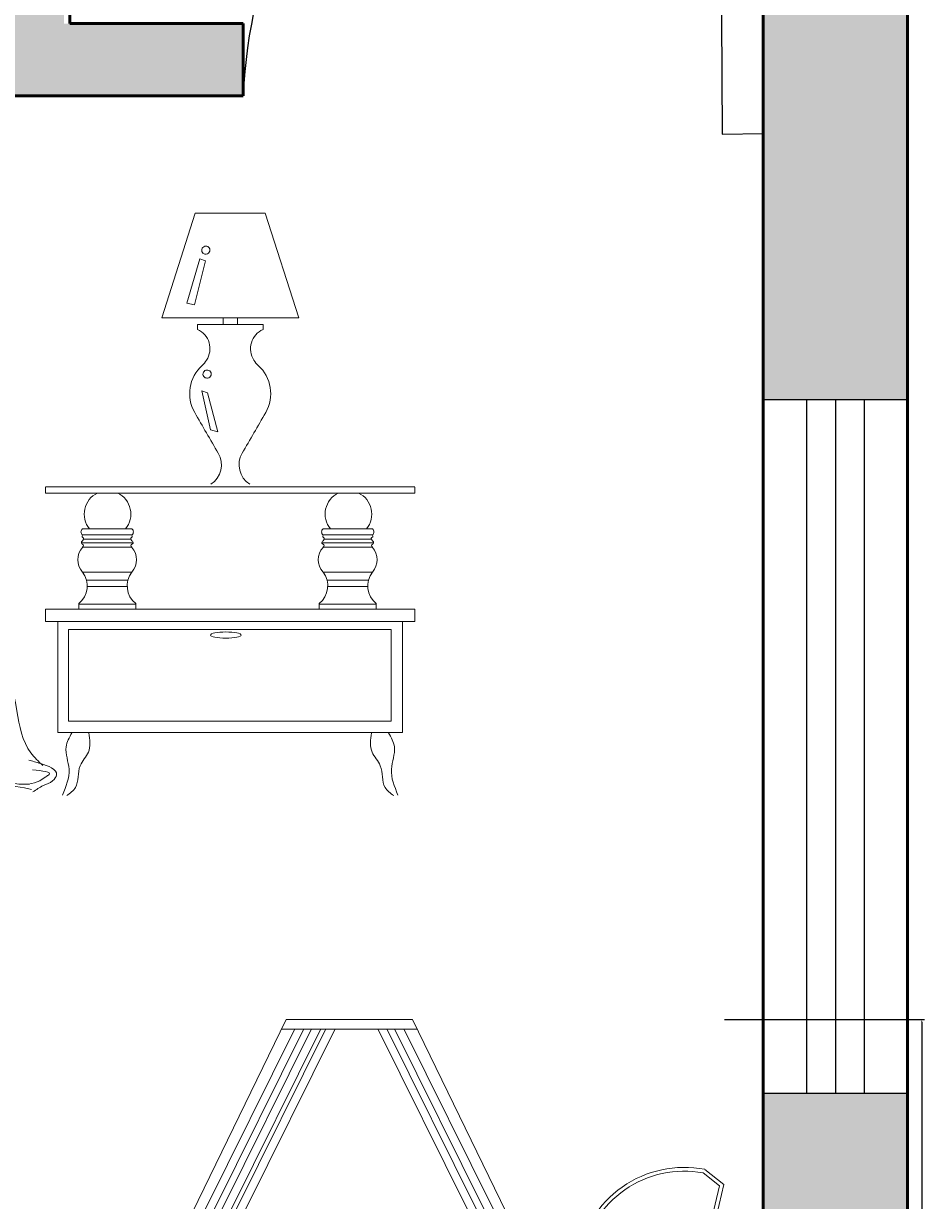
# Model space of a CAD drawing. Units: inches. Extents: x 1771 to 3025, y 319 to 889.
# Tile 11 of 35: x 2040 to 2102, y 713 to 795. Entities that reach past the tile are written whole.
import ezdxf

# ---------------------------------------------------------------- set-up
doc = ezdxf.new("R2010")
doc.units = ezdxf.units.IN
doc.header["$MEASUREMENT"] = 0
doc.set_wipeout_variables(frame=1)
for name, color, linetype, lineweight in [('A-ANNO-DIMS', 2, 'Continuous', 18), ('A-DOOR', 4, 'Continuous', 25), ('A-FURN', 8, 'Continuous', 18), ('A-GLAZ', 40, 'Continuous', 25), ('A-WALL', 7, 'Continuous', 50), ('A-WALL-PATT', 254, 'Continuous', 13)]:
    doc.layers.add(name, color=color, linetype=linetype, lineweight=lineweight)
doc.styles.get("Standard").update_dxf_attribs({"font": 'arial.ttf'})
doc.dimstyles.get("Standard").update_dxf_attribs({"dimtxt": 0.18, "dimasz": 0.18, "dimexe": 0.18, "dimexo": 0.0625, "dimgap": 0.09, "dimtad": 0, "dimtih": 1, "dimtoh": 1, "dimdec": 4, "dimzin": 0, "dimdsep": 46, "dimtxsty": 'Standard', "dimcen": 0.09, "dimadec": 0, "dimazin": 0, "dimtfac": 1, "dimtdec": 4, "dimtofl": 0, "dimtmove": 0, "dimatfit": 3, "dimfxl": 1, "dimtolj": 1, "dimtzin": 0, "dimarcsym": 0})

# ---------------------------------------------------------------- blocks, each defined once
blk = doc.blocks.new('A$C3F6F0378')
for p, q in [((2294.6, 774.2), (2348.7, 943.6)), ((2462.2, 943.6), (2348.7, 943.6)), ((2516.4, 774.2), (2462.2, 943.6)), ((2335.1, 797.8), (2356.3, 869.3)), ((2365.5, 866.2), (2347.3, 794.8)), ((2356.3, 869.3), (2365.5, 866.2)), ((2347.3, 794.8), (2335.1, 797.8)), ((2516.4, 774.2), (2294.6, 774.2)), ((2352.3, 763), (2352.3, 755.2)), ((2352.3, 763), (2352.3, 755.2)), ((2458.6, 763), (2352.3, 763)), ((2393.8, 774.2), (2393.8, 763)), ((2417.1, 763), (2393.8, 763)), ((2417.1, 774.2), (2417.1, 763)), ((2458.6, 763), (2458.6, 755.2)), ((2458.6, 763), (2458.6, 755.2)), ((2359.5, 655.6), (2368.6, 652.5)), ((2373.2, 592.3), (2359.5, 655.6)), ((2368.6, 652.5), (2385.4, 589.2)), ((2385.4, 589.2), (2373.2, 592.3)), ((2704.5, 500), (2106.1, 500)), ((2106.1, 499.7), (2106.1, 489.7)), ((2704.5, 499.7), (2704.5, 489.7)), ((2704.5, 490), (2106.1, 490)), ((2246.1, 432.2), (2166.1, 432.2)), ((2246.1, 432.2), (2166.1, 432.2)), ((2246.1, 422.2), (2166.1, 422.2)), ((2635.9, 432.2), (2555.9, 432.2)), ((2635.9, 432.2), (2555.9, 432.2)), ((2635.9, 422.2), (2555.9, 422.2)), ((2248, 409.3), (2164.1, 409.3)), ((2246.1, 402.2), (2166.1, 402.2)), ((2244.2, 415.4), (2167.9, 415.4)), ((2637.9, 409.3), (2554, 409.3)), ((2635.9, 402.2), (2555.9, 402.2)), ((2634.1, 415.4), (2557.7, 415.4)), ((2246.1, 362.2), (2166.1, 362.2)), ((2239.7, 349.2), (2172.4, 349.2)), ((2635.9, 362.2), (2555.9, 362.2)), ((2629.6, 349.2), (2562.2, 349.2)), ((2238.5, 338.7), (2173.6, 338.7)), ((2628.4, 338.7), (2563.5, 338.7)), ((2159.8, 311), (2159.8, 302.2)), ((2252.3, 310.3), (2159.8, 310.3)), ((2252.3, 311), (2252.3, 302.2)), ((2549.7, 311), (2549.7, 302.2)), ((2642.2, 310.3), (2549.7, 310.3)), ((2642.2, 311), (2642.2, 302.2)), ((2106.1, 302.2), (2106.1, 282.2)), ((2704.5, 302.2), (2106.1, 302.2)), ((2186.1, 302.2), (2226.1, 302.2)), ((2186.1, 302.2), (2236.1, 302.2)), ((2575.9, 302.2), (2615.9, 302.2)), ((2575.9, 302.2), (2625.9, 302.2)), ((2704.5, 282.2), (2704.5, 302.2)), ((2704.5, 282.2), (2106.1, 282.2)), ((2126.1, 282.2), (2126.1, 102.2)), ((2143.3, 268.9), (2666.3, 268.9)), ((2143.3, 120.8), (2143.3, 268.9)), ((2666.3, 268.9), (2666.3, 120.8)), ((2684.5, 102.2), (2684.5, 282.2)), ((2666.3, 120.8), (2143.3, 120.8)), ((2126.1, 102.2), (2684.5, 102.2))]:
    blk.add_line(p, q)
for centre, radius, start, end in [((2365.7, 883.6), 6.48, 168.6084, 233.2112), ((2365.7, 883.6), 6.49, 104.0344, 168.6084), ((2365.7, 883.5), 6.42, 233.2112, 255.9722), ((2366.1, 883.6), 6.51, 78.6968, 107.1924), ((2365.7, 883.8), 6.69, 255.9722, 278.2688), ((2365.7, 883.9), 6.81, 278.2688, 342.9026), ((2366.1, 883.7), 6.5, 50.1648, 78.6968), ((2366.2, 883.8), 6.35, 342.9026, 50.1648), ((2338.7, 724.1), 33.9, 326.6744, 66.3416), ((2472.2, 724.1), 33.9, 113.6584, 213.3256), ((2337, 722.3), 34.4, 312.0366, 330.6067), ((2473.8, 722.3), 34.4, 209.3933, 227.9634), ((2401.2, 651.2), 61.5, 132.0366, 209.8723), ((2367.7, 682.8), 6.49, 104.0344, 168.6084), ((2368.1, 682.9), 6.51, 78.6968, 107.1924), ((2368.1, 682.9), 6.5, 50.1648, 78.6968), ((2368.2, 683), 6.35, 342.9026, 50.1648), ((2409.6, 651.2), 61.5, 330.1277, 47.9634), ((2367.7, 682.8), 6.48, 168.6084, 233.2112), ((2367.7, 682.8), 6.42, 233.2112, 255.9722), ((2367.8, 683), 6.69, 255.9722, 278.2688), ((2367.8, 683.1), 6.81, 278.2688, 342.9026), ((11218.8, 5715.8), 10230.1, 209.87228, 210.29853), ((-6408, 5715.8), 10230.1, 329.70147, 330.12772), ((2353.9, 535.9), 37.3, 302.5427, 30.2985), ((2457, 535.9), 37.3, 149.7015, 237.4573), ((2206.6, 456.1), 37.8, 115.9414, 219.2084), ((2206.6, 456.1), 37.8, 320.7916, 64.0586), ((2597, 456.1), 37.8, 115.9414, 219.2084), ((2597, 456.1), 37.8, 320.7916, 64.0586), ((2169.8, 427.2), 6.24, 126.78, 233.22), ((2242.3, 427.2), 6.24, 306.78, 53.22), ((2559.7, 427.2), 6.24, 126.78, 233.22), ((2632.2, 427.2), 6.24, 306.78, 53.22), ((2188.1, 382.2), 29.7, 137.7452, 222.2548), ((2224, 382.2), 29.7, 317.7452, 42.2548), ((2577.9, 382.2), 29.7, 137.7452, 222.2548), ((2613.9, 382.2), 29.7, 317.7452, 42.2548), ((2136.7, 339.8), 37, 308.7547, 37.2668), ((2275.4, 339.8), 37, 142.7332, 231.2453), ((2526.5, 339.8), 37, 308.7547, 37.2668), ((2665.3, 339.8), 37, 142.7332, 231.2453)]:
    blk.add_arc(centre, radius, start, end)
blk.add_ellipse((2398.3, 260.1), major_axis=(25, 0), ratio=0.2)
at = {"ltscale": 5}
for points, knots in [([(2101.8, 49), (2094.8, 55.3), (2069.8, 78.1), (2053.9, 172), (2031.7, 287.1), (2023.3, 445.1), (1887.5, 475), (1637.7, 455.3), (1416.4, 458.5), (1314.5, 461.4)], [0, 0, 0, 0, 28.320233, 100.953775, 269.820348, 420.691469, 489.161544, 656.134073, 940.569207, 940.569207, 940.569207, 940.569207]), ([(2079, 57.4), (2084.9, 55.8), (2100.2, 51.8), (2131, 40.6), (2116.7, 21.1), (2101.3, 16.6), (2091, 9.7), (2085.5, 5.9)], [0, 0, 0, 0, 19.937155, 51.57724, 63.193909, 80.21631, 100.09061, 100.09061, 100.09061, 100.09061]), ([(2080.3, 18.4), (2075.6, 18.3), (2062.2, 17.9), (2030.9, 24.9), (1978.8, 41.9), (1919.5, 46.5), (1879.3, 50.9), (1863, 53.1), (1860.4, 51), (1859.9, 50.7)], [0, 0, 0, 0, 14.447875, 40.468341, 96.220884, 181.018327, 216.046098, 224.609189, 226.185962, 226.185962, 226.185962, 226.185962]), ([(2084.9, 41.8), (2100.9, 40.1), (2120.5, 38.1), (2104.4, 29.7), (2095.5, 21.9), (2085.1, 19.8), (2078.6, 18.4)], [0, 0, 0, 0, 28.05485, 34.289435, 45.980108, 65.027556, 65.027556, 65.027556, 65.027556]), ([(2083.5, 9.9), (2082, 10.3), (2061.3, 15.5), (2017.8, 18.7), (1949.9, 25.1), (1893.7, 17), (1853.5, 15.4), (1840.4, 23.1), (1835.5, 26)], [590.079786, 590.079786, 590.079786, 590.079786, 594.646549, 651.888327, 725.747367, 797.841373, 826.274406, 843.189267, 843.189267, 843.189267, 843.189267])]:
    blk.add_open_spline(points, degree=3, knots=knots, dxfattribs=at)
for points, knots in [([(2166.1, 422.2), (2165.6, 421), (2164.6, 418.8), (2169.4, 417.1), (2166.2, 412.9), (2162.3, 408.7), (2169.1, 405.7), (2166.9, 403.1), (2166.1, 402.2)], [0, 0, 0, 0, 3.125, 6.207289, 10.622222, 14.901958, 20.470919, 23.596268, 23.596268, 23.596268, 23.596268]), ([(2246, 422.2), (2246.5, 421), (2247.5, 418.8), (2242.7, 417.1), (2245.9, 412.9), (2249.8, 408.7), (2243, 405.7), (2245.2, 403.1), (2246, 402.2)], [0, 0, 0, 0, 3.125, 6.207289, 10.622222, 14.901958, 20.470919, 23.596268, 23.596268, 23.596268, 23.596268]), ([(2555.9, 422.2), (2555.5, 421), (2554.5, 418.8), (2559.3, 417.1), (2556.1, 412.9), (2552.2, 408.7), (2559, 405.7), (2556.7, 403.1), (2555.9, 402.2)], [0, 0, 0, 0, 3.125, 6.207289, 10.622222, 14.901958, 20.470919, 23.596268, 23.596268, 23.596268, 23.596268]), ([(2635.9, 422.2), (2636.4, 421), (2637.3, 418.8), (2632.5, 417.1), (2635.8, 412.9), (2639.7, 408.7), (2632.8, 405.7), (2635.1, 403.1), (2635.9, 402.2)], [0, 0, 0, 0, 3.125, 6.207289, 10.622222, 14.901958, 20.470919, 23.596268, 23.596268, 23.596268, 23.596268]), ([(2148.9, 101.6), (2144.7, 94.2), (2134.2, 75.7), (2149.9, 40.1), (2139.4, 14.7), (2133.7, 0.9)], [0, 0, 0, 0, 24.696996, 61.099524, 104.177437, 104.177437, 104.177437, 104.177437]), ([(2176.5, 101.6), (2178, 90.6), (2180.7, 70.5), (2155.8, 47.4), (2161.8, 15.4), (2145.9, 4), (2140.4, 0)], [0, 0, 0, 0, 31.35672, 56.935761, 92.890491, 112.386558, 112.386558, 112.386558, 112.386558]), ([(2634.4, 101.6), (2632.9, 90.6), (2630.2, 70.5), (2655.1, 47.4), (2649.1, 15.4), (2665, 4), (2670.5, 0)], [0, 0, 0, 0, 31.35672, 56.935761, 92.890491, 112.386558, 112.386558, 112.386558, 112.386558]), ([(2662, 101.6), (2666.2, 94.2), (2676.7, 75.7), (2661, 40.1), (2671.5, 14.7), (2677.2, 0.9)], [0, 0, 0, 0, 24.696996, 61.099524, 104.177437, 104.177437, 104.177437, 104.177437])]:
    blk.add_open_spline(points, degree=3, knots=knots)
blk = doc.blocks.new('A$C425441F1')
for points in [[(1639.3, 0), (1667.3, 0), (1667.3, 55.3), (1748.6, 55.3), (1748.6, 807.4), (1761.1, 860.7), (1735.7, 880.7), (1703.4, 883.3), (1675.8, 879.6), (1656.2, 873.5), (1635.2, 863.3), (1619.6, 852.6), (1605.1, 839.5), (1596.7, 829.9), (1583.2, 810), (1573.2, 788.1), (1567.6, 767.7), (1566.5, 761.6), (1541.6, 750.9), (1510.7, 736.6), (1488.3, 725.3), (1464.5, 712.2), (1433.4, 693.6), (1409.1, 677.8), (1389.7, 664.2), (1388.2, 683.8), (1383.3, 700), (1376.2, 712), (1365.5, 723.2), (1352, 731.8), (1342.1, 735.4), (1331.7, 738.6), (1325, 742.7), (1317.7, 750.9), (1314.2, 758.8), (1312.9, 767.9), (1315.6, 780.8), (1321.1, 788.9), (1323.4, 793.7), (1323.6, 797.2), (1323.1, 800), (1320.5, 804.5), (1317.8, 806.7), (1317.8, 807.1), (1478.8, 807.1), (1345.8, 1080.7), (1177.3, 1080.7), (1044.3, 807.1), (1211.1, 807.1), (1211.1, 806.7), (1207.8, 803.9), (1205.8, 800.4), (1205.1, 796.3), (1207.6, 788.9), (1211.4, 783.4), (1213.5, 778.7), (1215.3, 769.8), (1215.1, 763.9), (1214.1, 759), (1208.8, 748.5), (1201.9, 741.7), (1195.3, 738), (1185.9, 735.4), (1176, 731.7), (1166.8, 726.4), (1159.9, 720.8), (1156.8, 717.7), (1149.3, 708.1), (1145.7, 701.6), (1143.6, 696.9), (1138.7, 669.7), (1138.7, 651.6), (1140.7, 631.8), (1142.6, 621.6), (1148.5, 600.5), (1162.8, 569), (1176.9, 547.8), (1188.6, 534.2), (1200, 523), (983, 523), (977.7, 522.3), (971.8, 519.6), (965.5, 512.8), (963.3, 506.8), (963, 503), (974.8, 503), (974.8, 3), (1013, 3), (1013, 103), (1053.6, 103), (1052.7, 96.1), (1051.6, 86.5), (1049.3, 63.6), (1048.6, 55.3), (1130.1, 55.3), (1130.1, 0), (1157.9, 0), (1174.1, 55.3), (1623.1, 55.6)], [(778.6, 0), (750.6, 0), (750.6, 50.4), (141.4, 50.4), (141.4, 0), (113.4, 0), (98.1, 50.4), (0, 50.4), (0, 590.4), (3.6, 609.1), (14.7, 633.7), (36.6, 658.7), (60.6, 673.3), (86.6, 680.5), (100.5, 681.5), (107.8, 698), (118.3, 717), (136.4, 751.3), (159.1, 779.5), (188.4, 803.6), (213.2, 817.4), (239.4, 827.1), (258.7, 831.4), (276, 833.4), (301.1, 842.1), (332.2, 850.9), (368.4, 858.6), (403.3, 863.5), (432.7, 865.8), (472.6, 866.2), (499.3, 864.8), (525, 862.1), (551.9, 857.9), (572.9, 853.6), (591.1, 849.1), (612.6, 842.8), (648, 830.4), (661.5, 823.7), (679.5, 815.2), (707.5, 798.2), (726.7, 783.3), (755.4, 754.4), (773.7, 729.8), (788.1, 704.9), (796.6, 686.1), (798.5, 681.2), (818, 677.9), (833.5, 672.3), (851.7, 661.6), (864.4, 650.3), (878.3, 632.1), (887.5, 611.7), (891.4, 595.2), (892, 590.4), (892, 50.4), (793.9, 50.4)]]:
    blk.add_wipeout(points)
for p, q in [((1044.3, 807.1), (1177.3, 1080.7)), ((1177.3, 1080.7), (1044.3, 807.1)), ((1188.8, 1068), (1069.3, 827.4)), ((1201.1, 1068), (1081.6, 827.4)), ((1211.2, 1068), (1091.7, 827.4)), ((1223.5, 1068), (1104, 827.4)), ((1230.5, 1068), (1110.9, 827.4)), ((1242.8, 1068), (1123.2, 827.4)), ((1171, 1067.8), (1351.9, 1067.8)), ((1177.3, 1080.7), (1345.8, 1080.7)), ((1345.8, 1080.7), (1177.3, 1080.7)), ((1299.6, 1068), (1419.2, 827.4)), ((1311.9, 1068), (1431.5, 827.4)), ((1322, 1068), (1441.5, 827.4)), ((1334.3, 1068), (1453.8, 827.4)), ((1345.8, 1080.7), (1478.8, 807.1)), ((1478.8, 807.1), (1345.8, 1080.7)), ((1735.7, 880.7), (1761.1, 860.7)), ((1733.6, 876.1), (1755.5, 858.7)), ((1744.1, 810.1), (1755.5, 858.7)), ((1748.6, 807.4), (1761.1, 860.7))]:
    blk.add_line(p, q)
for radius, start, end in [(143.6, 79.0486, 171.2543), (138.6, 79.5487, 170.0411)]:
    blk.add_arc((1708.4, 739.8), radius, start, end)
blk = doc.blocks.new('DOOR-35')
blk.add_lwpolyline([(35.881, 36.185), (32.957, 36.297), (33.165, 0), (36, 0.055)], close=True)
blk.add_arc((35.225, 1.111), 35.259, 93.68792, 177.49253)
blk = doc.blocks.new('WIN-48')
for p, q in [((0, 0), (0, 10)), ((48, 0), (48, 10)), ((0, 7), (48, 7)), ((0, 5), (48, 5)), ((0, 3), (48, 3))]:
    blk.add_line(p, q)
blk = doc.blocks.new('*D39')
at = {"layer": 'A-ANNO-DIMS', "color": 0, "lineweight": -2, "transparency": 16777216}
for p, q in [((2088.055, 725.724), (2101.883, 725.724)), ((2101.703, 725.544), (2101.703, 697.861)), ((2101.703, 669.814), (2101.703, 697.497)), ((2088.055, 669.634), (2101.883, 669.634))]:
    blk.add_line(p, q, dxfattribs=at)
at = {"layer": 'A-ANNO-DIMS', "color": 0, "transparency": 16777216}
for points in [[(2101.673, 725.544), (2101.733, 725.544), (2101.703, 725.724)], [(2101.673, 669.814), (2101.733, 669.814), (2101.703, 669.634)]]:
    blk.add_solid(points, dxfattribs=at)
at = {"layer": 'Defpoints', "color": 0, "transparency": 16777216}
for p in [(2087.993, 725.724), (2101.703, 725.724), (2087.993, 669.634)]:
    blk.add_point(p, dxfattribs=at)
at = {"layer": 'A-ANNO-DIMS', "color": 0, "transparency": 16777216, "insert": (2101.703, 697.679), "char_height": 0.18, "attachment_point": 5}
blk.add_mtext('\\A1;56 TYP.', dxfattribs=at)

msp = doc.modelspace()

# ---------------------------------------------------------------- hatches: boundary and pattern name
at = {"layer": 'A-WALL-PATT'}
h = msp.add_hatch(color=256, dxfattribs=at)
h.dxf.hatch_style = 1
h.paths.add_polyline_path([(1870.724, 888.634), (1799.724, 888.634), (1799.724, 878.634), (1870.724, 878.634)])
h.paths.add_polyline_path([(1968.767, 888.634), (1918.724, 888.634), (1918.724, 878.634), (1941.724, 878.634), (1941.724, 830.634), (1946.724, 830.634), (1946.724, 878.634), (1968.767, 878.634)])
h.paths.add_polyline_path([(2059.676, 888.634), (2016.767, 888.634), (2016.767, 878.634), (2037.724, 878.634), (2037.724, 794.634), (1941.724, 794.634), (1941.724, 758.634), (1941.724, 664.634), (1946.724, 664.634), (1946.724, 712), (1946.724, 789.634), (2054.724, 789.634), (2054.724, 794.634), (2042.325, 794.634), (2042.325, 798.62), (2042.325, 835.497), (2042.724, 878.634), (2059.676, 878.634)])
h.paths.add_polyline_path([(2100.724, 888.634), (2077.676, 888.634), (2077.676, 878.634), (2090.724, 878.634), (2090.724, 789.634), (2090.724, 768.608), (2100.724, 768.608)])
h.paths.add_polyline_path([(2100.724, 720.608), (2090.724, 720.608), (2090.724, 669.634), (1982.724, 669.634), (1982.724, 664.634), (2001.724, 664.634), (2001.724, 652.634), (2006.724, 652.634), (2006.724, 664.634), (2049.518, 664.634, -0.385549), (2050.522, 664.634), (2090.724, 664.634), (2090.724, 649.173), (2100.724, 649.173)])
edge = h.paths.add_edge_path()
edge.add_line((2100.724, 631.173), (2090.724, 631.173))
edge.add_line((2090.724, 631.173), (2090.724, 616.634))
edge.add_line((2090.724, 616.634), (2001.724, 616.634))
edge.add_line((2001.724, 616.634), (1982.724, 616.634))
edge.add_line((1982.724, 616.634), (1982.724, 611.634))
edge.add_line((1982.724, 611.634), (2024.672, 611.634))
edge.add_spline(control_points=[(2024.672, 611.634), (2027.581, 612.871), (2030.014, 613.313), (2032.469, 613.716)], knot_values=[484.321569, 484.321569, 484.321569, 484.321569, 625.498764, 625.498764, 625.498764, 625.498764], degree=3, periodic=0)
edge.add_line((2032.469, 613.716), (2033.205, 613.716))
edge.add_spline(control_points=[(2033.205, 613.716), (2035.66, 613.313), (2039.461, 612.871), (2042.204, 611.634)], knot_values=[484.321569, 484.321569, 484.321569, 484.321569, 625.498764, 625.498764, 625.498764, 625.498764], degree=3, periodic=0)
edge.add_line((2042.204, 611.634), (2090.724, 611.634))
edge.add_line((2090.724, 611.634), (2090.724, 581.106))
edge.add_line((2090.724, 581.106), (2100.724, 581.106))
edge.add_line((2100.724, 581.106), (2100.724, 631.173))
h.paths.add_polyline_path([(2100.724, 533.106), (2090.724, 533.106), (2090.724, 479.634), (1946.724, 479.634), (1946.724, 616.634), (1936.724, 616.634), (1936.724, 543.634), (1845.724, 543.634), (1845.724, 533.634), (1936.724, 533.634), (1936.724, 469.634), (2090.724, 469.634), (2090.724, 452.762), (2100.724, 452.762)])
h.paths.add_polyline_path([(2100.724, 404.762), (2090.724, 404.762), (2090.724, 393.634), (1936.724, 393.634), (1936.724, 383.634), (2100.724, 383.634)])
h.paths.add_polyline_path([(1905.724, 758.634), (1835.47, 758.634), (1835.47, 758.634), (1813.444, 758.634), (1809.724, 758.634), (1809.724, 842.589, -0.008336), (1808.421, 842.634), (1799.724, 842.634), (1799.724, 690.584), (1809.724, 690.584), (1809.724, 753.634), (1905.724, 753.634)])
h.paths.add_polyline_path([(1809.724, 642.584), (1799.724, 642.584), (1799.724, 533.634), (1809.724, 533.634), (1809.724, 581)])

# ---------------------------------------------------------------- linework, layer by layer
at = {"layer": 'A-WALL'}
for p, q in [((2100.724, 383.634), (2100.724, 888.432)), ((2042.724, 794.634), (2042.724, 878.634)), ((2090.724, 789.634), (2090.724, 878.634)), ((2054.724, 794.634), (2042.724, 794.634)), ((2054.724, 789.634), (2054.724, 794.634)), ((2054.724, 789.634), (1946.724, 789.634)), ((2090.724, 669.634), (2090.724, 789.634))]:
    msp.add_line(p, q, dxfattribs=at)

# ---------------------------------------------------------------- block references
at = {"layer": 'A-DOOR'}
msp.add_blockref('DOOR-35', (2054.724, 786.98), dxfattribs=at)
at = {"layer": 'A-FURN', "xscale": 0.0427162254345911, "yscale": 0.0427162254345911, "zscale": 0.0427162254345911}
msp.add_blockref('A$C3F6F0378', (1951.078, 741.208), dxfattribs=at)
at = {"layer": 'A-GLAZ', "rotation": 270.0000000000007}
msp.add_blockref('WIN-48', (2090.724, 768.608), dxfattribs=at)

# ---------------------------------------------------------------- next in the draw order: block references
at = {"layer": 'A-FURN', "xscale": 0.0519011286993662, "yscale": 0.0519011286993662, "zscale": 0.0519011286993662}
msp.add_blockref('A$C425441F1', (1996.592, 669.634), dxfattribs=at)

# ---------------------------------------------------------------- next in the draw order: dimensions: what is measured, and where the dimension line sits
at = {"layer": 'A-ANNO-DIMS'}
dim = msp.add_linear_dim(base=(2101.703, 725.724), p1=(2087.993, 669.634), p2=(2087.993, 725.724), angle=90, text='<> TYP.', dimstyle='Standard', override={"dimdec": 0, "dimrnd": 0, "dimzin": 0, "dimlunit": 2}, dxfattribs=at)
dim.commit()
dim.dimension.update_dxf_attribs({"geometry": '*D39', "text_midpoint": (2101.703, 697.679)})

doc.saveas('drawing.dxf')
